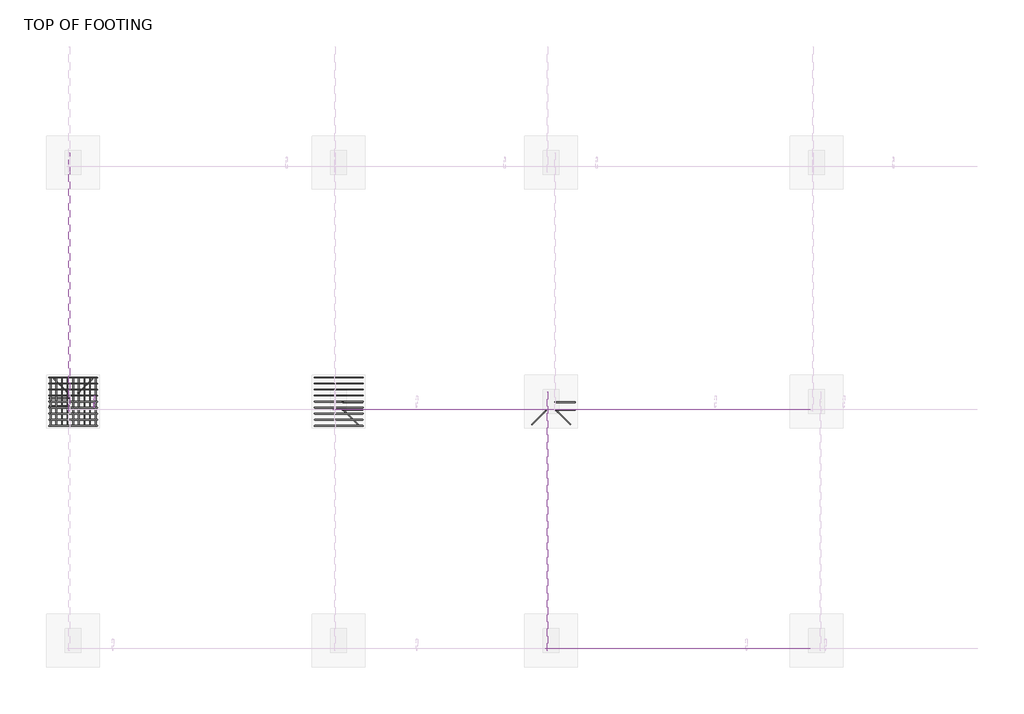
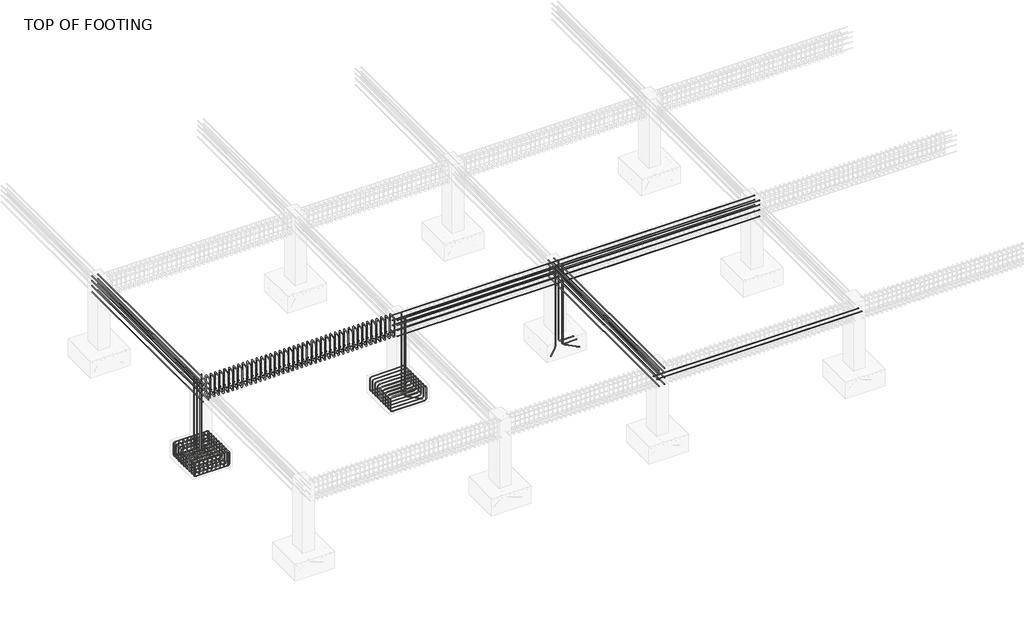
# One storey, part 4 of 13: 32 reinforcing bars.
"""IFC4 building model written with IfcOpenShell, lengths in millimetres."""

from ifc_helpers import new_model, si_unit, point, frame, origin, place, context, project, spatial, polyline, circle_curve, trimmed, segment, composite_curve, source, transform, mapped, element, save
from ifc_brep_helpers import swept_disk

model = new_model("IFC4")

# Units and contexts
model_context = context("Model", 3, world=origin())
ifc_project = project(units=[si_unit("LENGTHUNIT", "METRE", prefix="MILLI")], contexts=[model_context])

# Site, building, storey
site = spatial("IfcSite", under=ifc_project)
building = spatial("IfcBuilding", under=site)
storey = spatial("IfcBuildingStorey", under=building, Name="TOP OF FOOTING", Elevation=-1828.8)

# Reinforcing bars
placement = place(None, origin())
reinforcing_bar_shape = source(origin(), model_context, "Body", "SolidModel", [
    swept_disk(composite_curve([segment(polyline([(-12666.6498378, 8486.1851908, -2049.322685), (-12666.6498378, 8486.1851908, -2196.622685)]), True, "CONTINUOUS"), segment(trimmed(circle_curve(frame((-12712.9998378, 8486.1851908, -2196.622685), z_axis=(0.0, 1.0, 0.0), x_axis=(46.350000000000364, 0.0, 0.0)), 46.35), [point((-12666.6498378, 8486.1851908, -2196.622685))], [point((-12712.9998378, 8486.1851908, -2242.972685))], True, "CARTESIAN"), True, "CONTINUOUS"), segment(polyline([(-12712.9998378, 8486.1851908, -2242.972685), (-13527.5998378, 8486.1851908, -2242.972685)]), True, "CONTINUOUS"), segment(trimmed(circle_curve(frame((-13527.5998378, 8486.1851908, -2196.622685), z_axis=(0.0, 1.0, 0.0), x_axis=(0.0, 0.0, -46.350000000000364)), 46.35), [point((-13527.5998378, 8486.1851908, -2242.972685))], [point((-13573.9498378, 8486.1851908, -2196.622685))], True, "CARTESIAN"), True, "CONTINUOUS"), segment(polyline([(-13573.9498378, 8486.1851908, -2196.622685), (-13573.9498378, 8486.1851908, -2049.322685)]), True, "CONTINUOUS")], self_intersect=False), 6.35),
])
element("IfcReinforcingBar", 1, at=placement, inside=storey, context=model_context, shape_type="MappedRepresentation", body=[
    mapped(reinforcing_bar_shape, transform((0.0, 0.0, 0.0), x_axis=(1.0, 0.0, 0.0), y_axis=(0.0, 1.0, 0.0), z_axis=(0.0, 0.0, 1.0))),
    mapped(reinforcing_bar_shape, transform((0.0, -113.4125, 0.0), x_axis=(1.0, 0.0, 0.0), y_axis=(0.0, 1.0, 0.0), z_axis=(0.0, 0.0, 1.0))),
    mapped(reinforcing_bar_shape, transform((0.0, -226.825, 0.0), x_axis=(1.0, 0.0, 0.0), y_axis=(0.0, 1.0, 0.0), z_axis=(0.0, 0.0, 1.0))),
    mapped(reinforcing_bar_shape, transform((0.0, -340.2375, 0.0), x_axis=(1.0, 0.0, 0.0), y_axis=(0.0, 1.0, 0.0), z_axis=(0.0, 0.0, 1.0))),
    mapped(reinforcing_bar_shape, transform((0.0, -453.65, 0.0), x_axis=(1.0, 0.0, 0.0), y_axis=(0.0, 1.0, 0.0), z_axis=(0.0, 0.0, 1.0))),
    mapped(reinforcing_bar_shape, transform((0.0, -567.0625, 0.0), x_axis=(1.0, 0.0, 0.0), y_axis=(0.0, 1.0, 0.0), z_axis=(0.0, 0.0, 1.0))),
    mapped(reinforcing_bar_shape, transform((0.0, -680.475, 0.0), x_axis=(1.0, 0.0, 0.0), y_axis=(0.0, 1.0, 0.0), z_axis=(0.0, 0.0, 1.0))),
    mapped(reinforcing_bar_shape, transform((0.0, -793.8875, 0.0), x_axis=(1.0, 0.0, 0.0), y_axis=(0.0, 1.0, 0.0), z_axis=(0.0, 0.0, 1.0))),
    mapped(reinforcing_bar_shape, transform((0.0, -907.3, 0.0), x_axis=(1.0, 0.0, 0.0), y_axis=(0.0, 1.0, 0.0), z_axis=(0.0, 0.0, 1.0))),
])
reinforcing_bar_2_shape = source(origin(), model_context, "Body", "SolidModel", [
    swept_disk(composite_curve([segment(polyline([(-13573.9498378, 8486.1851908, -2051.3998363), (-13573.9498378, 8486.1851908, -1904.0998363)]), True, "CONTINUOUS"), segment(trimmed(circle_curve(frame((-13527.5998378, 8486.1851908, -1904.0998363), z_axis=(0.0, 1.0, 0.0), x_axis=(-46.350000000000364, 0.0, 0.0)), 46.35), [point((-13573.9498378, 8486.1851908, -1904.0998363))], [point((-13527.5998378, 8486.1851908, -1857.7498363))], True, "CARTESIAN"), True, "CONTINUOUS"), segment(polyline([(-13527.5998378, 8486.1851908, -1857.7498363), (-12712.9998378, 8486.1851908, -1857.7498363)]), True, "CONTINUOUS"), segment(trimmed(circle_curve(frame((-12712.9998378, 8486.1851908, -1904.0998363), z_axis=(0.0, 1.0, 0.0), x_axis=(0.0, 0.0, 46.350000000000136)), 46.35), [point((-12712.9998378, 8486.1851908, -1857.7498363))], [point((-12666.6498378, 8486.1851908, -1904.0998363))], True, "CARTESIAN"), True, "CONTINUOUS"), segment(polyline([(-12666.6498378, 8486.1851908, -1904.0998363), (-12666.6498378, 8486.1851908, -2051.3998363)]), True, "CONTINUOUS")], self_intersect=False), 6.35),
])
element("IfcReinforcingBar", 2, at=placement, inside=storey, context=model_context, shape_type="MappedRepresentation", body=[
    mapped(reinforcing_bar_2_shape, transform((0.0, 0.0, 0.0), x_axis=(1.0, 0.0, 0.0), y_axis=(0.0, 1.0, 0.0), z_axis=(0.0, 0.0, 1.0))),
    mapped(reinforcing_bar_2_shape, transform((0.0, -113.4125, 0.0), x_axis=(1.0, 0.0, 0.0), y_axis=(0.0, 1.0, 0.0), z_axis=(0.0, 0.0, 1.0))),
    mapped(reinforcing_bar_2_shape, transform((0.0, -226.825, 0.0), x_axis=(1.0, 0.0, 0.0), y_axis=(0.0, 1.0, 0.0), z_axis=(0.0, 0.0, 1.0))),
    mapped(reinforcing_bar_2_shape, transform((0.0, -340.2375, 0.0), x_axis=(1.0, 0.0, 0.0), y_axis=(0.0, 1.0, 0.0), z_axis=(0.0, 0.0, 1.0))),
    mapped(reinforcing_bar_2_shape, transform((0.0, -453.65, 0.0), x_axis=(1.0, 0.0, 0.0), y_axis=(0.0, 1.0, 0.0), z_axis=(0.0, 0.0, 1.0))),
    mapped(reinforcing_bar_2_shape, transform((0.0, -567.0625, 0.0), x_axis=(1.0, 0.0, 0.0), y_axis=(0.0, 1.0, 0.0), z_axis=(0.0, 0.0, 1.0))),
    mapped(reinforcing_bar_2_shape, transform((0.0, -680.475, 0.0), x_axis=(1.0, 0.0, 0.0), y_axis=(0.0, 1.0, 0.0), z_axis=(0.0, 0.0, 1.0))),
    mapped(reinforcing_bar_2_shape, transform((0.0, -793.8875, 0.0), x_axis=(1.0, 0.0, 0.0), y_axis=(0.0, 1.0, 0.0), z_axis=(0.0, 0.0, 1.0))),
    mapped(reinforcing_bar_2_shape, transform((0.0, -907.3, 0.0), x_axis=(1.0, 0.0, 0.0), y_axis=(0.0, 1.0, 0.0), z_axis=(0.0, 0.0, 1.0))),
])
reinforcing_bar_3_shape = source(origin(), model_context, "Body", "SolidModel", [
    swept_disk(composite_curve([segment(polyline([(-13542.4641345, 8486.1851908, -2025.081839), (-13542.4641345, 8486.1851908, -2172.381839)]), True, "CONTINUOUS"), segment(trimmed(circle_curve(frame((-13542.4641345, 8439.8351908, -2172.381839), z_axis=(-1.0, 0.0, 0.0), x_axis=(0.0, 46.350000000000364, 0.0)), 46.35), [point((-13542.4641345, 8486.1851908, -2172.381839))], [point((-13542.4641345, 8439.8351908, -2218.731839))], True, "CARTESIAN"), True, "CONTINUOUS"), segment(polyline([(-13542.4641345, 8439.8351908, -2218.731839), (-13542.4641345, 7625.2351908, -2218.731839)]), True, "CONTINUOUS"), segment(trimmed(circle_curve(frame((-13542.4641345, 7625.2351908, -2172.381839), z_axis=(-1.0, 0.0, 0.0), x_axis=(0.0, 0.0, -46.34999999999991)), 46.35), [point((-13542.4641345, 7625.2351908, -2218.731839))], [point((-13542.4641345, 7578.8851908, -2172.381839))], True, "CARTESIAN"), True, "CONTINUOUS"), segment(polyline([(-13542.4641345, 7578.8851908, -2172.381839), (-13542.4641345, 7578.8851908, -2025.081839)]), True, "CONTINUOUS")], self_intersect=False), 6.35),
])
element("IfcReinforcingBar", 3, at=placement, inside=storey, context=model_context, shape_type="MappedRepresentation", body=[
    mapped(reinforcing_bar_3_shape, transform((0.0, 0.0, 0.0), x_axis=(1.0, 0.0, 0.0), y_axis=(0.0, 1.0, 0.0), z_axis=(0.0, 0.0, 1.0))),
    mapped(reinforcing_bar_3_shape, transform((105.924033, 0.0, 0.0), x_axis=(1.0, 0.0, 0.0), y_axis=(0.0, 1.0, 0.0), z_axis=(0.0, 0.0, 1.0))),
    mapped(reinforcing_bar_3_shape, transform((211.8480661, 0.0, 0.0), x_axis=(1.0, 0.0, 0.0), y_axis=(0.0, 1.0, 0.0), z_axis=(0.0, 0.0, 1.0))),
    mapped(reinforcing_bar_3_shape, transform((317.7720991, 0.0, 0.0), x_axis=(1.0, 0.0, 0.0), y_axis=(0.0, 1.0, 0.0), z_axis=(0.0, 0.0, 1.0))),
    mapped(reinforcing_bar_3_shape, transform((423.6961321, 0.0, 0.0), x_axis=(1.0, 0.0, 0.0), y_axis=(0.0, 1.0, 0.0), z_axis=(0.0, 0.0, 1.0))),
    mapped(reinforcing_bar_3_shape, transform((529.6201652, 0.0, 0.0), x_axis=(1.0, 0.0, 0.0), y_axis=(0.0, 1.0, 0.0), z_axis=(0.0, 0.0, 1.0))),
    mapped(reinforcing_bar_3_shape, transform((635.5441982, 0.0, 0.0), x_axis=(1.0, 0.0, 0.0), y_axis=(0.0, 1.0, 0.0), z_axis=(0.0, 0.0, 1.0))),
    mapped(reinforcing_bar_3_shape, transform((741.4682312, 0.0, 0.0), x_axis=(1.0, 0.0, 0.0), y_axis=(0.0, 1.0, 0.0), z_axis=(0.0, 0.0, 1.0))),
    mapped(reinforcing_bar_3_shape, transform((847.3922643, 0.0, 0.0), x_axis=(1.0, 0.0, 0.0), y_axis=(0.0, 1.0, 0.0), z_axis=(0.0, 0.0, 1.0))),
])
reinforcing_bar_4_shape = source(origin(), model_context, "Body", "SolidModel", [
    swept_disk(composite_curve([segment(polyline([(-12695.0718702, 8486.1851908, -2069.0990329), (-12695.0718702, 8486.1851908, -1921.7990329)]), True, "CONTINUOUS"), segment(trimmed(circle_curve(frame((-12695.0718702, 8439.8351908, -1921.7990329), z_axis=(1.0, 0.0, 0.0), x_axis=(0.0, 46.350000000000364, 0.0)), 46.35), [point((-12695.0718702, 8486.1851908, -1921.7990329))], [point((-12695.0718702, 8439.8351908, -1875.4490329))], True, "CARTESIAN"), True, "CONTINUOUS"), segment(polyline([(-12695.0718702, 8439.8351908, -1875.4490329), (-12695.0718702, 7625.2351908, -1875.4490329)]), True, "CONTINUOUS"), segment(trimmed(circle_curve(frame((-12695.0718702, 7625.2351908, -1921.7990329), z_axis=(1.0, 0.0, 0.0), x_axis=(0.0, 0.0, 46.34999999999991)), 46.35), [point((-12695.0718702, 7625.2351908, -1875.4490329))], [point((-12695.0718702, 7578.8851908, -1921.7990329))], True, "CARTESIAN"), True, "CONTINUOUS"), segment(polyline([(-12695.0718702, 7578.8851908, -1921.7990329), (-12695.0718702, 7578.8851908, -2069.0990329)]), True, "CONTINUOUS")], self_intersect=False), 6.35),
])
element("IfcReinforcingBar", 4, at=placement, inside=storey, context=model_context, shape_type="MappedRepresentation", body=[
    mapped(reinforcing_bar_4_shape, transform((0.0, 0.0, 0.0), x_axis=(1.0, 0.0, 0.0), y_axis=(0.0, 1.0, 0.0), z_axis=(0.0, 0.0, 1.0))),
    mapped(reinforcing_bar_4_shape, transform((-105.924033, 0.0, 0.0), x_axis=(1.0, 0.0, 0.0), y_axis=(0.0, 1.0, 0.0), z_axis=(0.0, 0.0, 1.0))),
    mapped(reinforcing_bar_4_shape, transform((-211.8480661, 0.0, 0.0), x_axis=(1.0, 0.0, 0.0), y_axis=(0.0, 1.0, 0.0), z_axis=(0.0, 0.0, 1.0))),
    mapped(reinforcing_bar_4_shape, transform((-317.7720991, 0.0, 0.0), x_axis=(1.0, 0.0, 0.0), y_axis=(0.0, 1.0, 0.0), z_axis=(0.0, 0.0, 1.0))),
    mapped(reinforcing_bar_4_shape, transform((-423.6961321, 0.0, 0.0), x_axis=(1.0, 0.0, 0.0), y_axis=(0.0, 1.0, 0.0), z_axis=(0.0, 0.0, 1.0))),
    mapped(reinforcing_bar_4_shape, transform((-529.6201652, 0.0, 0.0), x_axis=(1.0, 0.0, 0.0), y_axis=(0.0, 1.0, 0.0), z_axis=(0.0, 0.0, 1.0))),
    mapped(reinforcing_bar_4_shape, transform((-635.5441982, 0.0, 0.0), x_axis=(1.0, 0.0, 0.0), y_axis=(0.0, 1.0, 0.0), z_axis=(0.0, 0.0, 1.0))),
    mapped(reinforcing_bar_4_shape, transform((-741.4682312, 0.0, 0.0), x_axis=(1.0, 0.0, 0.0), y_axis=(0.0, 1.0, 0.0), z_axis=(0.0, 0.0, 1.0))),
    mapped(reinforcing_bar_4_shape, transform((-847.3922643, 0.0, 0.0), x_axis=(1.0, 0.0, 0.0), y_axis=(0.0, 1.0, 0.0), z_axis=(0.0, 0.0, 1.0))),
])
reinforcing_bar_5_shape = source(origin(), model_context, "Body", "SolidModel", [
    swept_disk(composite_curve([segment(polyline([(-7666.6498378, 8486.1851908, -2049.322685), (-7666.6498378, 8486.1851908, -2196.622685)]), True, "CONTINUOUS"), segment(trimmed(circle_curve(frame((-7712.9998378, 8486.1851908, -2196.622685), z_axis=(0.0, 1.0, 0.0), x_axis=(46.350000000000364, 0.0, 0.0)), 46.35), [point((-7666.6498378, 8486.1851908, -2196.622685))], [point((-7712.9998378, 8486.1851908, -2242.972685))], True, "CARTESIAN"), True, "CONTINUOUS"), segment(polyline([(-7712.9998378, 8486.1851908, -2242.972685), (-8527.5998378, 8486.1851908, -2242.972685)]), True, "CONTINUOUS"), segment(trimmed(circle_curve(frame((-8527.5998378, 8486.1851908, -2196.622685), z_axis=(0.0, 1.0, 0.0), x_axis=(0.0, 0.0, -46.350000000000364)), 46.35), [point((-8527.5998378, 8486.1851908, -2242.972685))], [point((-8573.9498378, 8486.1851908, -2196.622685))], True, "CARTESIAN"), True, "CONTINUOUS"), segment(polyline([(-8573.9498378, 8486.1851908, -2196.622685), (-8573.9498378, 8486.1851908, -2049.322685)]), True, "CONTINUOUS")], self_intersect=False), 6.35),
])
element("IfcReinforcingBar", 5, at=placement, inside=storey, context=model_context, shape_type="MappedRepresentation", body=[
    mapped(reinforcing_bar_5_shape, transform((0.0, 0.0, 0.0), x_axis=(1.0, 0.0, 0.0), y_axis=(0.0, 1.0, 0.0), z_axis=(0.0, 0.0, 1.0))),
    mapped(reinforcing_bar_5_shape, transform((0.0, -113.4125, 0.0), x_axis=(1.0, 0.0, 0.0), y_axis=(0.0, 1.0, 0.0), z_axis=(0.0, 0.0, 1.0))),
    mapped(reinforcing_bar_5_shape, transform((0.0, -226.825, 0.0), x_axis=(1.0, 0.0, 0.0), y_axis=(0.0, 1.0, 0.0), z_axis=(0.0, 0.0, 1.0))),
    mapped(reinforcing_bar_5_shape, transform((0.0, -340.2375, 0.0), x_axis=(1.0, 0.0, 0.0), y_axis=(0.0, 1.0, 0.0), z_axis=(0.0, 0.0, 1.0))),
    mapped(reinforcing_bar_5_shape, transform((0.0, -453.65, 0.0), x_axis=(1.0, 0.0, 0.0), y_axis=(0.0, 1.0, 0.0), z_axis=(0.0, 0.0, 1.0))),
    mapped(reinforcing_bar_5_shape, transform((0.0, -567.0625, 0.0), x_axis=(1.0, 0.0, 0.0), y_axis=(0.0, 1.0, 0.0), z_axis=(0.0, 0.0, 1.0))),
    mapped(reinforcing_bar_5_shape, transform((0.0, -680.475, 0.0), x_axis=(1.0, 0.0, 0.0), y_axis=(0.0, 1.0, 0.0), z_axis=(0.0, 0.0, 1.0))),
    mapped(reinforcing_bar_5_shape, transform((0.0, -793.8875, 0.0), x_axis=(1.0, 0.0, 0.0), y_axis=(0.0, 1.0, 0.0), z_axis=(0.0, 0.0, 1.0))),
    mapped(reinforcing_bar_5_shape, transform((0.0, -907.3, 0.0), x_axis=(1.0, 0.0, 0.0), y_axis=(0.0, 1.0, 0.0), z_axis=(0.0, 0.0, 1.0))),
])
reinforcing_bar_6_shape = source(origin(), model_context, "Body", "SolidModel", [
    swept_disk(composite_curve([segment(polyline([(-8573.9498378, 8486.1851908, -2051.3998363), (-8573.9498378, 8486.1851908, -1904.0998363)]), True, "CONTINUOUS"), segment(trimmed(circle_curve(frame((-8527.5998378, 8486.1851908, -1904.0998363), z_axis=(0.0, 1.0, 0.0), x_axis=(-46.350000000000364, 0.0, 0.0)), 46.35), [point((-8573.9498378, 8486.1851908, -1904.0998363))], [point((-8527.5998378, 8486.1851908, -1857.7498363))], True, "CARTESIAN"), True, "CONTINUOUS"), segment(polyline([(-8527.5998378, 8486.1851908, -1857.7498363), (-7712.9998378, 8486.1851908, -1857.7498363)]), True, "CONTINUOUS"), segment(trimmed(circle_curve(frame((-7712.9998378, 8486.1851908, -1904.0998363), z_axis=(0.0, 1.0, 0.0), x_axis=(0.0, 0.0, 46.350000000000136)), 46.35), [point((-7712.9998378, 8486.1851908, -1857.7498363))], [point((-7666.6498378, 8486.1851908, -1904.0998363))], True, "CARTESIAN"), True, "CONTINUOUS"), segment(polyline([(-7666.6498378, 8486.1851908, -1904.0998363), (-7666.6498378, 8486.1851908, -2051.3998363)]), True, "CONTINUOUS")], self_intersect=False), 6.35),
])
element("IfcReinforcingBar", 6, at=placement, inside=storey, context=model_context, shape_type="MappedRepresentation", body=[
    mapped(reinforcing_bar_6_shape, transform((0.0, 0.0, 0.0), x_axis=(1.0, 0.0, 0.0), y_axis=(0.0, 1.0, 0.0), z_axis=(0.0, 0.0, 1.0))),
    mapped(reinforcing_bar_6_shape, transform((0.0, -113.4125, 0.0), x_axis=(1.0, 0.0, 0.0), y_axis=(0.0, 1.0, 0.0), z_axis=(0.0, 0.0, 1.0))),
    mapped(reinforcing_bar_6_shape, transform((0.0, -226.825, 0.0), x_axis=(1.0, 0.0, 0.0), y_axis=(0.0, 1.0, 0.0), z_axis=(0.0, 0.0, 1.0))),
    mapped(reinforcing_bar_6_shape, transform((0.0, -340.2375, 0.0), x_axis=(1.0, 0.0, 0.0), y_axis=(0.0, 1.0, 0.0), z_axis=(0.0, 0.0, 1.0))),
    mapped(reinforcing_bar_6_shape, transform((0.0, -453.65, 0.0), x_axis=(1.0, 0.0, 0.0), y_axis=(0.0, 1.0, 0.0), z_axis=(0.0, 0.0, 1.0))),
    mapped(reinforcing_bar_6_shape, transform((0.0, -567.0625, 0.0), x_axis=(1.0, 0.0, 0.0), y_axis=(0.0, 1.0, 0.0), z_axis=(0.0, 0.0, 1.0))),
    mapped(reinforcing_bar_6_shape, transform((0.0, -680.475, 0.0), x_axis=(1.0, 0.0, 0.0), y_axis=(0.0, 1.0, 0.0), z_axis=(0.0, 0.0, 1.0))),
    mapped(reinforcing_bar_6_shape, transform((0.0, -793.8875, 0.0), x_axis=(1.0, 0.0, 0.0), y_axis=(0.0, 1.0, 0.0), z_axis=(0.0, 0.0, 1.0))),
    mapped(reinforcing_bar_6_shape, transform((0.0, -907.3, 0.0), x_axis=(1.0, 0.0, 0.0), y_axis=(0.0, 1.0, 0.0), z_axis=(0.0, 0.0, 1.0))),
])
reinforcing_bar_7_shape = source(origin(), model_context, "Body", "SolidModel", [
    swept_disk(composite_curve([segment(polyline([(-4044.6810723, 8023.2621018, -40.0), (-4044.6810723, 8023.2621018, -2147.4714407)]), True, "CONTINUOUS"), segment(trimmed(circle_curve(frame((-3998.3310723, 8023.2621018, -2147.4714407), z_axis=(0.0, -1.0, 0.0), x_axis=(-46.34999999999991, 0.0, 0.0)), 46.35), [point((-4044.6810723, 8023.2621018, -2147.4714407))], [point((-3998.3310723, 8023.2621018, -2193.8214407))], True, "CARTESIAN"), True, "CONTINUOUS"), segment(polyline([(-3998.3310723, 8023.2621018, -2193.8214407), (-3667.4997506, 8023.2621018, -2193.8214407)]), True, "CONTINUOUS")], self_intersect=False), 6.35),
])
element("IfcReinforcingBar", 7, at=placement, inside=storey, context=model_context, shape_type="MappedRepresentation", body=[
    mapped(reinforcing_bar_7_shape, transform((0.0, 0.0, 0.0), x_axis=(1.0, 0.0, 0.0), y_axis=(0.0, 1.0, 0.0), z_axis=(0.0, 0.0, 1.0))),
    mapped(reinforcing_bar_7_shape, transform((0.0, -144.620853, 0.0), x_axis=(1.0, 0.0, 0.0), y_axis=(0.0, 1.0, 0.0), z_axis=(0.0, 0.0, 1.0))),
])
element("IfcReinforcingBar", 8, at=placement, inside=storey, context=model_context, shape_type="SolidModel", body=[
    swept_disk(composite_curve([segment(polyline([(-4024.6810723, 7868.8851908, -40.0), (-4024.6810723, 7868.8851908, -2147.4714407)]), True, "CONTINUOUS"), segment(trimmed(circle_curve(frame((-3991.906673, 7836.1107915, -2147.4714407), z_axis=(-0.7071067811865542, -0.7071067811865408, 0.0), x_axis=(-32.774399299999914, 32.77439929999946, 0.0)), 46.35), [point((-4024.6810723, 7868.8851908, -2147.4714407))], [point((-3991.906673, 7836.1107915, -2193.8214407))], True, "CARTESIAN"), True, "CONTINUOUS"), segment(polyline([(-3991.906673, 7836.1107915, -2193.8214407), (-3757.973602, 7602.1777205, -2193.8214407)]), True, "CONTINUOUS")], self_intersect=False), 6.35),
])
element("IfcReinforcingBar", 9, at=placement, inside=storey, context=model_context, shape_type="SolidModel", body=[
    swept_disk(composite_curve([segment(polyline([(-4215.9186034, 7868.8851908, -40.0), (-4215.9186034, 7868.8851908, -2147.4714407)]), True, "CONTINUOUS"), segment(trimmed(circle_curve(frame((-4248.6930027, 7836.1107915, -2147.4714407), z_axis=(-0.7071067811865339, 0.7071067811865611, 0.0), x_axis=(32.77439929999946, 32.77439929999946, 0.0)), 46.35), [point((-4215.9186034, 7868.8851908, -2147.4714407))], [point((-4248.6930027, 7836.1107915, -2193.8214407))], True, "CARTESIAN"), True, "CONTINUOUS"), segment(polyline([(-4248.6930027, 7836.1107915, -2193.8214407), (-4482.6260737, 7602.1777205, -2193.8214407)]), True, "CONTINUOUS")], self_intersect=False), 6.35),
])
reinforcing_bar_8_shape = source(origin(), model_context, "Body", "SolidModel", [
    swept_disk(composite_curve([segment(polyline([(-8044.6810723, 8023.2621018, -40.0), (-8044.6810723, 8023.2621018, -2147.4714407)]), True, "CONTINUOUS"), segment(trimmed(circle_curve(frame((-7998.3310723, 8023.2621018, -2147.4714407), z_axis=(0.0, -1.0, 0.0), x_axis=(-46.349999999999454, 0.0, 0.0)), 46.35), [point((-8044.6810723, 8023.2621018, -2147.4714407))], [point((-7998.3310723, 8023.2621018, -2193.8214407))], True, "CARTESIAN"), True, "CONTINUOUS"), segment(polyline([(-7998.3310723, 8023.2621018, -2193.8214407), (-7667.4997506, 8023.2621018, -2193.8214407)]), True, "CONTINUOUS")], self_intersect=False), 6.35),
])
element("IfcReinforcingBar", 10, at=placement, inside=storey, context=model_context, shape_type="MappedRepresentation", body=[
    mapped(reinforcing_bar_8_shape, transform((0.0, 0.0, 0.0), x_axis=(1.0, 0.0, 0.0), y_axis=(0.0, 1.0, 0.0), z_axis=(0.0, 0.0, 1.0))),
    mapped(reinforcing_bar_8_shape, transform((0.0, -144.620853, 0.0), x_axis=(1.0, 0.0, 0.0), y_axis=(0.0, 1.0, 0.0), z_axis=(0.0, 0.0, 1.0))),
])
element("IfcReinforcingBar", 11, at=placement, inside=storey, context=model_context, shape_type="SolidModel", body=[
    swept_disk(composite_curve([segment(polyline([(-8024.6810723, 7868.8851908, -40.0), (-8024.6810723, 7868.8851908, -2147.4714407)]), True, "CONTINUOUS"), segment(trimmed(circle_curve(frame((-7991.906673, 7836.1107915, -2147.4714407), z_axis=(-0.7071067811865542, -0.7071067811865408, 0.0), x_axis=(-32.77439929999946, 32.77439929999946, 0.0)), 46.35), [point((-8024.6810723, 7868.8851908, -2147.4714407))], [point((-7991.906673, 7836.1107915, -2193.8214407))], True, "CARTESIAN"), True, "CONTINUOUS"), segment(polyline([(-7991.906673, 7836.1107915, -2193.8214407), (-7757.973602, 7602.1777205, -2193.8214407)]), True, "CONTINUOUS")], self_intersect=False), 6.35),
])
element("IfcReinforcingBar", 12, at=placement, inside=storey, context=model_context, shape_type="SolidModel", body=[
    swept_disk(composite_curve([segment(polyline([(-13024.6810723, 8196.1851908, -40.0), (-13024.6810723, 8196.1851908, -2147.4714407)]), True, "CONTINUOUS"), segment(trimmed(circle_curve(frame((-12991.906673, 8228.9595901, -2147.4714407), z_axis=(0.7071067811865476, -0.7071067811865475, 0.0), x_axis=(-32.77439930000037, -32.77439929999855, 0.0)), 46.35), [point((-13024.6810723, 8196.1851908, -2147.4714407))], [point((-12991.906673, 8228.9595901, -2193.8214407))], True, "CARTESIAN"), True, "CONTINUOUS"), segment(polyline([(-12991.906673, 8228.9595901, -2193.8214407), (-12757.973602, 8462.8926611, -2193.8214407)]), True, "CONTINUOUS")], self_intersect=False), 6.35),
])
element("IfcReinforcingBar", 13, at=placement, inside=storey, context=model_context, shape_type="SolidModel", body=[
    swept_disk(composite_curve([segment(polyline([(-13215.9186034, 8196.1851908, -40.0), (-13215.9186034, 8196.1851908, -2147.4714407)]), True, "CONTINUOUS"), segment(trimmed(circle_curve(frame((-13248.6930027, 8228.9595901, -2147.4714407), z_axis=(0.7071067811865679, 0.7071067811865271, 0.0), x_axis=(32.77439930000037, -32.77439929999855, 0.0)), 46.35), [point((-13215.9186034, 8196.1851908, -2147.4714407))], [point((-13248.6930027, 8228.9595901, -2193.8214407))], True, "CARTESIAN"), True, "CONTINUOUS"), segment(polyline([(-13248.6930027, 8228.9595901, -2193.8214407), (-13482.6260737, 8462.8926611, -2193.8214407)]), True, "CONTINUOUS")], self_intersect=False), 6.35),
])
reinforcing_bar_9_shape = source(origin(), model_context, "Body", "SolidModel", [
    swept_disk(composite_curve([segment(polyline([(-13195.9186034, 8098.2621018, -40.0), (-13195.9186034, 8098.2621018, -2147.4714407)]), True, "CONTINUOUS"), segment(trimmed(circle_curve(frame((-13242.2686034, 8098.2621018, -2147.4714407), z_axis=(0.0, 1.0, 0.0), x_axis=(46.350000000000364, 0.0, 0.0)), 46.35), [point((-13195.9186034, 8098.2621018, -2147.4714407))], [point((-13242.2686034, 8098.2621018, -2193.8214407))], True, "CARTESIAN"), True, "CONTINUOUS"), segment(polyline([(-13242.2686034, 8098.2621018, -2193.8214407), (-13573.0999251, 8098.2621018, -2193.8214407)]), True, "CONTINUOUS")], self_intersect=False), 6.35),
])
element("IfcReinforcingBar", 14, at=placement, inside=storey, context=model_context, shape_type="MappedRepresentation", body=[
    mapped(reinforcing_bar_9_shape, transform((0.0, 0.0, 0.0), x_axis=(1.0, 0.0, 0.0), y_axis=(0.0, 1.0, 0.0), z_axis=(0.0, 0.0, 1.0))),
    mapped(reinforcing_bar_9_shape, transform((0.0, -144.620853, 0.0), x_axis=(1.0, 0.0, 0.0), y_axis=(0.0, 1.0, 0.0), z_axis=(0.0, 0.0, 1.0))),
])
reinforcing_bar_10_shape = source(origin(), model_context, "Body", "SolidModel", [
    swept_disk(composite_curve([segment(polyline([(-4192.6754021, 3347.5351908, -87.6047527), (-4192.6754021, 8217.5351908, -87.6047527)]), True, "CONTINUOUS")], self_intersect=False), 6.35),
])
element("IfcReinforcingBar", 15, at=placement, inside=storey, context=model_context, shape_type="MappedRepresentation", body=[
    mapped(reinforcing_bar_10_shape, transform((0.0, 0.0, 0.0), x_axis=(1.0, 0.0, 0.0), y_axis=(0.0, 1.0, 0.0), z_axis=(0.0, 0.0, 1.0))),
    mapped(reinforcing_bar_10_shape, transform((144.710816, 0.0, 0.0), x_axis=(1.0, 0.0, 0.0), y_axis=(0.0, 1.0, 0.0), z_axis=(0.0, 0.0, 1.0))),
])
reinforcing_bar_11_shape = source(origin(), model_context, "Body", "SolidModel", [
    swept_disk(composite_curve([segment(polyline([(-4192.6754021, 3347.5351908, -212.6047527), (-4192.6754021, 8217.5351908, -212.6047527)]), True, "CONTINUOUS")], self_intersect=False), 6.35),
])
element("IfcReinforcingBar", 16, at=placement, inside=storey, context=model_context, shape_type="MappedRepresentation", body=[
    mapped(reinforcing_bar_11_shape, transform((0.0, 0.0, 0.0), x_axis=(1.0, 0.0, 0.0), y_axis=(0.0, 1.0, 0.0), z_axis=(0.0, 0.0, 1.0))),
    mapped(reinforcing_bar_11_shape, transform((144.710816, 0.0, 0.0), x_axis=(1.0, 0.0, 0.0), y_axis=(0.0, 1.0, 0.0), z_axis=(0.0, 0.0, 1.0))),
])
reinforcing_bar_12_shape = source(origin(), model_context, "Body", "SolidModel", [
    swept_disk(composite_curve([segment(polyline([(-4192.6754021, 3347.5351908, -517.6047527), (-4192.6754021, 8217.5351908, -517.6047527)]), True, "CONTINUOUS")], self_intersect=False), 6.35),
])
element("IfcReinforcingBar", 17, at=placement, inside=storey, context=model_context, shape_type="MappedRepresentation", body=[
    mapped(reinforcing_bar_12_shape, transform((0.0, 0.0, 0.0), x_axis=(1.0, 0.0, 0.0), y_axis=(0.0, 1.0, 0.0), z_axis=(0.0, 0.0, 1.0))),
    mapped(reinforcing_bar_12_shape, transform((144.710816, 0.0, 0.0), x_axis=(1.0, 0.0, 0.0), y_axis=(0.0, 1.0, 0.0), z_axis=(0.0, 0.0, 1.0))),
])
reinforcing_bar_13_shape = source(origin(), model_context, "Body", "SolidModel", [
    swept_disk(composite_curve([segment(polyline([(-4192.6754021, 3347.5351908, -347.6047527), (-4192.6754021, 8217.5351908, -347.6047527)]), True, "CONTINUOUS")], self_intersect=False), 6.35),
])
element("IfcReinforcingBar", 18, at=placement, inside=storey, context=model_context, shape_type="MappedRepresentation", body=[
    mapped(reinforcing_bar_13_shape, transform((0.0, 0.0, 0.0), x_axis=(1.0, 0.0, 0.0), y_axis=(0.0, 1.0, 0.0), z_axis=(0.0, 0.0, 1.0))),
    mapped(reinforcing_bar_13_shape, transform((144.710816, 0.0, 0.0), x_axis=(1.0, 0.0, 0.0), y_axis=(0.0, 1.0, 0.0), z_axis=(0.0, 0.0, 1.0))),
])
reinforcing_bar_14_shape = source(origin(), model_context, "Body", "SolidModel", [
    swept_disk(composite_curve([segment(polyline([(-13192.6754021, 7847.5351908, -87.6047527), (-13192.6754021, 12717.5351908, -87.6047527)]), True, "CONTINUOUS")], self_intersect=False), 6.35),
])
element("IfcReinforcingBar", 19, at=placement, inside=storey, context=model_context, shape_type="MappedRepresentation", body=[
    mapped(reinforcing_bar_14_shape, transform((0.0, 0.0, 0.0), x_axis=(1.0, 0.0, 0.0), y_axis=(0.0, 1.0, 0.0), z_axis=(0.0, 0.0, 1.0))),
    mapped(reinforcing_bar_14_shape, transform((144.710816, 0.0, 0.0), x_axis=(1.0, 0.0, 0.0), y_axis=(0.0, 1.0, 0.0), z_axis=(0.0, 0.0, 1.0))),
])
reinforcing_bar_15_shape = source(origin(), model_context, "Body", "SolidModel", [
    swept_disk(composite_curve([segment(polyline([(-13192.6754021, 7847.5351908, -212.6047527), (-13192.6754021, 12717.5351908, -212.6047527)]), True, "CONTINUOUS")], self_intersect=False), 6.35),
])
element("IfcReinforcingBar", 20, at=placement, inside=storey, context=model_context, shape_type="MappedRepresentation", body=[
    mapped(reinforcing_bar_15_shape, transform((0.0, 0.0, 0.0), x_axis=(1.0, 0.0, 0.0), y_axis=(0.0, 1.0, 0.0), z_axis=(0.0, 0.0, 1.0))),
    mapped(reinforcing_bar_15_shape, transform((144.710816, 0.0, 0.0), x_axis=(1.0, 0.0, 0.0), y_axis=(0.0, 1.0, 0.0), z_axis=(0.0, 0.0, 1.0))),
])
reinforcing_bar_16_shape = source(origin(), model_context, "Body", "SolidModel", [
    swept_disk(composite_curve([segment(polyline([(-13192.6754021, 7847.5351908, -517.6047527), (-13192.6754021, 12717.5351908, -517.6047527)]), True, "CONTINUOUS")], self_intersect=False), 6.35),
])
element("IfcReinforcingBar", 21, at=placement, inside=storey, context=model_context, shape_type="MappedRepresentation", body=[
    mapped(reinforcing_bar_16_shape, transform((0.0, 0.0, 0.0), x_axis=(1.0, 0.0, 0.0), y_axis=(0.0, 1.0, 0.0), z_axis=(0.0, 0.0, 1.0))),
    mapped(reinforcing_bar_16_shape, transform((144.710816, 0.0, 0.0), x_axis=(1.0, 0.0, 0.0), y_axis=(0.0, 1.0, 0.0), z_axis=(0.0, 0.0, 1.0))),
])
reinforcing_bar_17_shape = source(origin(), model_context, "Body", "SolidModel", [
    swept_disk(composite_curve([segment(polyline([(-13192.6754021, 7847.5351908, -347.6047527), (-13192.6754021, 12717.5351908, -347.6047527)]), True, "CONTINUOUS")], self_intersect=False), 6.35),
])
element("IfcReinforcingBar", 22, at=placement, inside=storey, context=model_context, shape_type="MappedRepresentation", body=[
    mapped(reinforcing_bar_17_shape, transform((0.0, 0.0, 0.0), x_axis=(1.0, 0.0, 0.0), y_axis=(0.0, 1.0, 0.0), z_axis=(0.0, 0.0, 1.0))),
    mapped(reinforcing_bar_17_shape, transform((144.710816, 0.0, 0.0), x_axis=(1.0, 0.0, 0.0), y_axis=(0.0, 1.0, 0.0), z_axis=(0.0, 0.0, 1.0))),
])
reinforcing_bar_18_shape = source(origin(), model_context, "Body", "SolidModel", [
    swept_disk(composite_curve([segment(polyline([(-8276.6498378, 8071.2594254, -444.3886395), (-8276.6498378, 8127.0029884, -500.1322024)]), True, "CONTINUOUS"), segment(trimmed(circle_curve(frame((-8276.6498378, 8104.8351908, -522.3), z_axis=(-1.0, 0.0, 0.0), x_axis=(0.0, 22.167797599999176, 22.16779759999997)), 31.35), [point((-8276.6498378, 8127.0029884, -500.1322024))], [point((-8276.6498378, 8104.8351908, -553.65))], True, "CARTESIAN"), True, "CONTINUOUS"), segment(polyline([(-8276.6498378, 8104.8351908, -553.65), (-8276.6498378, 7960.2351908, -553.65)]), True, "CONTINUOUS"), segment(trimmed(circle_curve(frame((-8276.6498378, 7960.2351908, -522.3), z_axis=(-1.0, 0.0, 0.0), x_axis=(0.0, 0.0, -31.350000000000023)), 31.35), [point((-8276.6498378, 7960.2351908, -553.65))], [point((-8276.6498378, 7928.8851908, -522.3))], True, "CARTESIAN"), True, "CONTINUOUS"), segment(polyline([(-8276.6498378, 7928.8851908, -522.3), (-8276.6498378, 7928.8851908, -77.7)]), True, "CONTINUOUS"), segment(trimmed(circle_curve(frame((-8274.7328097, 7960.1765235, -77.7), z_axis=(-0.9981286353368323, 0.061149221750018364, 0.0), x_axis=(-1.917028099998788, -31.291332700000567, 0.0)), 31.35), [point((-8276.6498378, 7928.8851908, -77.7))], [point((-8274.7328097, 7960.1765235, -46.35))], True, "CARTESIAN"), True, "CONTINUOUS"), segment(polyline([(-8274.7328097, 7960.1765235, -46.35), (-8265.8668659, 8104.8938581, -46.35)]), True, "CONTINUOUS"), segment(trimmed(circle_curve(frame((-8265.8668659, 8104.8938581, -77.7), z_axis=(-0.9981286353368323, 0.061149221750018364, 0.0), x_axis=(0.0, 0.0, 31.35)), 31.35), [point((-8265.8668659, 8104.8938581, -46.35))], [point((-8263.9498378, 8136.1851908, -77.7))], True, "CARTESIAN"), True, "CONTINUOUS"), segment(polyline([(-8263.9498378, 8136.1851908, -77.7), (-8263.9498378, 8136.1851908, -522.3)]), True, "CONTINUOUS"), segment(trimmed(circle_curve(frame((-8263.9498378, 8104.8351908, -522.3), z_axis=(-1.0, 0.0, 0.0), x_axis=(0.0, 31.349999999999454, 0.0)), 31.35), [point((-8263.9498378, 8136.1851908, -522.3))], [point((-8263.9498378, 8082.6673932, -544.4677976))], True, "CARTESIAN"), True, "CONTINUOUS"), segment(polyline([(-8263.9498378, 8082.6673932, -544.4677976), (-8263.9498378, 8026.9238303, -488.7242346)]), True, "CONTINUOUS")], self_intersect=False), 6.35),
])
element("IfcReinforcingBar", 23, at=placement, inside=storey, context=model_context, shape_type="MappedRepresentation", body=[
    mapped(reinforcing_bar_18_shape, transform((0.0, 0.0, 0.0), x_axis=(1.0, 0.0, 0.0), y_axis=(0.0, 1.0, 0.0), z_axis=(0.0, 0.0, 1.0))),
    mapped(reinforcing_bar_18_shape, transform((-117.1825, 0.0, 0.0), x_axis=(1.0, 0.0, 0.0), y_axis=(0.0, 1.0, 0.0), z_axis=(0.0, 0.0, 1.0))),
    mapped(reinforcing_bar_18_shape, transform((-234.365, 0.0, 0.0), x_axis=(1.0, 0.0, 0.0), y_axis=(0.0, 1.0, 0.0), z_axis=(0.0, 0.0, 1.0))),
    mapped(reinforcing_bar_18_shape, transform((-351.5475, 0.0, 0.0), x_axis=(1.0, 0.0, 0.0), y_axis=(0.0, 1.0, 0.0), z_axis=(0.0, 0.0, 1.0))),
    mapped(reinforcing_bar_18_shape, transform((-468.73, 0.0, 0.0), x_axis=(1.0, 0.0, 0.0), y_axis=(0.0, 1.0, 0.0), z_axis=(0.0, 0.0, 1.0))),
    mapped(reinforcing_bar_18_shape, transform((-585.9125, 0.0, 0.0), x_axis=(1.0, 0.0, 0.0), y_axis=(0.0, 1.0, 0.0), z_axis=(0.0, 0.0, 1.0))),
    mapped(reinforcing_bar_18_shape, transform((-703.095, 0.0, 0.0), x_axis=(1.0, 0.0, 0.0), y_axis=(0.0, 1.0, 0.0), z_axis=(0.0, 0.0, 1.0))),
    mapped(reinforcing_bar_18_shape, transform((-820.2775, 0.0, 0.0), x_axis=(1.0, 0.0, 0.0), y_axis=(0.0, 1.0, 0.0), z_axis=(0.0, 0.0, 1.0))),
    mapped(reinforcing_bar_18_shape, transform((-937.46, 0.0, 0.0), x_axis=(1.0, 0.0, 0.0), y_axis=(0.0, 1.0, 0.0), z_axis=(0.0, 0.0, 1.0))),
    mapped(reinforcing_bar_18_shape, transform((-1054.6425, 0.0, 0.0), x_axis=(1.0, 0.0, 0.0), y_axis=(0.0, 1.0, 0.0), z_axis=(0.0, 0.0, 1.0))),
    mapped(reinforcing_bar_18_shape, transform((-1171.825, 0.0, 0.0), x_axis=(1.0, 0.0, 0.0), y_axis=(0.0, 1.0, 0.0), z_axis=(0.0, 0.0, 1.0))),
    mapped(reinforcing_bar_18_shape, transform((-1289.0075, 0.0, 0.0), x_axis=(1.0, 0.0, 0.0), y_axis=(0.0, 1.0, 0.0), z_axis=(0.0, 0.0, 1.0))),
    mapped(reinforcing_bar_18_shape, transform((-1406.19, 0.0, 0.0), x_axis=(1.0, 0.0, 0.0), y_axis=(0.0, 1.0, 0.0), z_axis=(0.0, 0.0, 1.0))),
    mapped(reinforcing_bar_18_shape, transform((-1523.3725, 0.0, 0.0), x_axis=(1.0, 0.0, 0.0), y_axis=(0.0, 1.0, 0.0), z_axis=(0.0, 0.0, 1.0))),
    mapped(reinforcing_bar_18_shape, transform((-1640.555, 0.0, 0.0), x_axis=(1.0, 0.0, 0.0), y_axis=(0.0, 1.0, 0.0), z_axis=(0.0, 0.0, 1.0))),
    mapped(reinforcing_bar_18_shape, transform((-1757.7375, 0.0, 0.0), x_axis=(1.0, 0.0, 0.0), y_axis=(0.0, 1.0, 0.0), z_axis=(0.0, 0.0, 1.0))),
    mapped(reinforcing_bar_18_shape, transform((-1874.92, 0.0, 0.0), x_axis=(1.0, 0.0, 0.0), y_axis=(0.0, 1.0, 0.0), z_axis=(0.0, 0.0, 1.0))),
    mapped(reinforcing_bar_18_shape, transform((-1992.1025, 0.0, 0.0), x_axis=(1.0, 0.0, 0.0), y_axis=(0.0, 1.0, 0.0), z_axis=(0.0, 0.0, 1.0))),
    mapped(reinforcing_bar_18_shape, transform((-2109.285, 0.0, 0.0), x_axis=(1.0, 0.0, 0.0), y_axis=(0.0, 1.0, 0.0), z_axis=(0.0, 0.0, 1.0))),
    mapped(reinforcing_bar_18_shape, transform((-2226.4675, 0.0, 0.0), x_axis=(1.0, 0.0, 0.0), y_axis=(0.0, 1.0, 0.0), z_axis=(0.0, 0.0, 1.0))),
    mapped(reinforcing_bar_18_shape, transform((-2343.65, 0.0, 0.0), x_axis=(1.0, 0.0, 0.0), y_axis=(0.0, 1.0, 0.0), z_axis=(0.0, 0.0, 1.0))),
    mapped(reinforcing_bar_18_shape, transform((-2460.8325, 0.0, 0.0), x_axis=(1.0, 0.0, 0.0), y_axis=(0.0, 1.0, 0.0), z_axis=(0.0, 0.0, 1.0))),
    mapped(reinforcing_bar_18_shape, transform((-2578.015, 0.0, 0.0), x_axis=(1.0, 0.0, 0.0), y_axis=(0.0, 1.0, 0.0), z_axis=(0.0, 0.0, 1.0))),
    mapped(reinforcing_bar_18_shape, transform((-2695.1975, 0.0, 0.0), x_axis=(1.0, 0.0, 0.0), y_axis=(0.0, 1.0, 0.0), z_axis=(0.0, 0.0, 1.0))),
    mapped(reinforcing_bar_18_shape, transform((-2812.38, 0.0, 0.0), x_axis=(1.0, 0.0, 0.0), y_axis=(0.0, 1.0, 0.0), z_axis=(0.0, 0.0, 1.0))),
    mapped(reinforcing_bar_18_shape, transform((-2929.5625, 0.0, 0.0), x_axis=(1.0, 0.0, 0.0), y_axis=(0.0, 1.0, 0.0), z_axis=(0.0, 0.0, 1.0))),
    mapped(reinforcing_bar_18_shape, transform((-3046.745, 0.0, 0.0), x_axis=(1.0, 0.0, 0.0), y_axis=(0.0, 1.0, 0.0), z_axis=(0.0, 0.0, 1.0))),
    mapped(reinforcing_bar_18_shape, transform((-3163.9275, 0.0, 0.0), x_axis=(1.0, 0.0, 0.0), y_axis=(0.0, 1.0, 0.0), z_axis=(0.0, 0.0, 1.0))),
    mapped(reinforcing_bar_18_shape, transform((-3281.11, 0.0, 0.0), x_axis=(1.0, 0.0, 0.0), y_axis=(0.0, 1.0, 0.0), z_axis=(0.0, 0.0, 1.0))),
    mapped(reinforcing_bar_18_shape, transform((-3398.2925, 0.0, 0.0), x_axis=(1.0, 0.0, 0.0), y_axis=(0.0, 1.0, 0.0), z_axis=(0.0, 0.0, 1.0))),
    mapped(reinforcing_bar_18_shape, transform((-3515.475, 0.0, 0.0), x_axis=(1.0, 0.0, 0.0), y_axis=(0.0, 1.0, 0.0), z_axis=(0.0, 0.0, 1.0))),
    mapped(reinforcing_bar_18_shape, transform((-3632.6575, 0.0, 0.0), x_axis=(1.0, 0.0, 0.0), y_axis=(0.0, 1.0, 0.0), z_axis=(0.0, 0.0, 1.0))),
    mapped(reinforcing_bar_18_shape, transform((-3749.84, 0.0, 0.0), x_axis=(1.0, 0.0, 0.0), y_axis=(0.0, 1.0, 0.0), z_axis=(0.0, 0.0, 1.0))),
    mapped(reinforcing_bar_18_shape, transform((-3867.0225, 0.0, 0.0), x_axis=(1.0, 0.0, 0.0), y_axis=(0.0, 1.0, 0.0), z_axis=(0.0, 0.0, 1.0))),
    mapped(reinforcing_bar_18_shape, transform((-3984.205, 0.0, 0.0), x_axis=(1.0, 0.0, 0.0), y_axis=(0.0, 1.0, 0.0), z_axis=(0.0, 0.0, 1.0))),
    mapped(reinforcing_bar_18_shape, transform((-4101.3875, 0.0, 0.0), x_axis=(1.0, 0.0, 0.0), y_axis=(0.0, 1.0, 0.0), z_axis=(0.0, 0.0, 1.0))),
    mapped(reinforcing_bar_18_shape, transform((-4218.57, 0.0, 0.0), x_axis=(1.0, 0.0, 0.0), y_axis=(0.0, 1.0, 0.0), z_axis=(0.0, 0.0, 1.0))),
    mapped(reinforcing_bar_18_shape, transform((-4335.7525, 0.0, 0.0), x_axis=(1.0, 0.0, 0.0), y_axis=(0.0, 1.0, 0.0), z_axis=(0.0, 0.0, 1.0))),
    mapped(reinforcing_bar_18_shape, transform((-4452.935, 0.0, 0.0), x_axis=(1.0, 0.0, 0.0), y_axis=(0.0, 1.0, 0.0), z_axis=(0.0, 0.0, 1.0))),
    mapped(reinforcing_bar_18_shape, transform((-4570.1175, 0.0, 0.0), x_axis=(1.0, 0.0, 0.0), y_axis=(0.0, 1.0, 0.0), z_axis=(0.0, 0.0, 1.0))),
    mapped(reinforcing_bar_18_shape, transform((-4687.3, 0.0, 0.0), x_axis=(1.0, 0.0, 0.0), y_axis=(0.0, 1.0, 0.0), z_axis=(0.0, 0.0, 1.0))),
])
reinforcing_bar_19_shape = source(origin(), model_context, "Body", "SolidModel", [
    swept_disk(composite_curve([segment(polyline([(-4010.2998378, 7885.1596265, -87.6047527), (-8230.2998378, 7885.1596265, -87.6047527)]), True, "CONTINUOUS")], self_intersect=False), 6.35),
])
element("IfcReinforcingBar", 24, at=placement, inside=storey, context=model_context, shape_type="MappedRepresentation", body=[
    mapped(reinforcing_bar_19_shape, transform((0.0, 0.0, 0.0), x_axis=(1.0, 0.0, 0.0), y_axis=(0.0, 1.0, 0.0), z_axis=(0.0, 0.0, 1.0))),
    mapped(reinforcing_bar_19_shape, transform((0.0, 219.710816, 0.0), x_axis=(1.0, 0.0, 0.0), y_axis=(0.0, 1.0, 0.0), z_axis=(0.0, 0.0, 1.0))),
])
reinforcing_bar_20_shape = source(origin(), model_context, "Body", "SolidModel", [
    swept_disk(composite_curve([segment(polyline([(-4010.2998378, 7885.1596265, -212.6047527), (-8230.2998378, 7885.1596265, -212.6047527)]), True, "CONTINUOUS")], self_intersect=False), 6.35),
])
element("IfcReinforcingBar", 25, at=placement, inside=storey, context=model_context, shape_type="MappedRepresentation", body=[
    mapped(reinforcing_bar_20_shape, transform((0.0, 0.0, 0.0), x_axis=(1.0, 0.0, 0.0), y_axis=(0.0, 1.0, 0.0), z_axis=(0.0, 0.0, 1.0))),
    mapped(reinforcing_bar_20_shape, transform((0.0, 219.710816, 0.0), x_axis=(1.0, 0.0, 0.0), y_axis=(0.0, 1.0, 0.0), z_axis=(0.0, 0.0, 1.0))),
])
reinforcing_bar_21_shape = source(origin(), model_context, "Body", "SolidModel", [
    swept_disk(composite_curve([segment(polyline([(-4010.2998378, 7885.1596265, -517.6047527), (-8230.2998378, 7885.1596265, -517.6047527)]), True, "CONTINUOUS")], self_intersect=False), 6.35),
])
element("IfcReinforcingBar", 26, at=placement, inside=storey, context=model_context, shape_type="MappedRepresentation", body=[
    mapped(reinforcing_bar_21_shape, transform((0.0, 0.0, 0.0), x_axis=(1.0, 0.0, 0.0), y_axis=(0.0, 1.0, 0.0), z_axis=(0.0, 0.0, 1.0))),
    mapped(reinforcing_bar_21_shape, transform((0.0, 219.710816, 0.0), x_axis=(1.0, 0.0, 0.0), y_axis=(0.0, 1.0, 0.0), z_axis=(0.0, 0.0, 1.0))),
])
reinforcing_bar_22_shape = source(origin(), model_context, "Body", "SolidModel", [
    swept_disk(composite_curve([segment(polyline([(-4010.2998378, 7885.1596265, -347.6047527), (-8230.2998378, 7885.1596265, -347.6047527)]), True, "CONTINUOUS")], self_intersect=False), 6.35),
])
element("IfcReinforcingBar", 27, at=placement, inside=storey, context=model_context, shape_type="MappedRepresentation", body=[
    mapped(reinforcing_bar_22_shape, transform((0.0, 0.0, 0.0), x_axis=(1.0, 0.0, 0.0), y_axis=(0.0, 1.0, 0.0), z_axis=(0.0, 0.0, 1.0))),
    mapped(reinforcing_bar_22_shape, transform((0.0, 219.710816, 0.0), x_axis=(1.0, 0.0, 0.0), y_axis=(0.0, 1.0, 0.0), z_axis=(0.0, 0.0, 1.0))),
])
reinforcing_bar_23_shape = source(origin(), model_context, "Body", "SolidModel", [
    swept_disk(composite_curve([segment(polyline([(989.7001622, 7885.1596265, -87.6047527), (-4230.2998378, 7885.1596265, -87.6047527)]), True, "CONTINUOUS")], self_intersect=False), 6.35),
])
element("IfcReinforcingBar", 28, at=placement, inside=storey, context=model_context, shape_type="MappedRepresentation", body=[
    mapped(reinforcing_bar_23_shape, transform((0.0, 0.0, 0.0), x_axis=(1.0, 0.0, 0.0), y_axis=(0.0, 1.0, 0.0), z_axis=(0.0, 0.0, 1.0))),
    mapped(reinforcing_bar_23_shape, transform((0.0, 219.710816, 0.0), x_axis=(1.0, 0.0, 0.0), y_axis=(0.0, 1.0, 0.0), z_axis=(0.0, 0.0, 1.0))),
])
reinforcing_bar_24_shape = source(origin(), model_context, "Body", "SolidModel", [
    swept_disk(composite_curve([segment(polyline([(989.7001622, 7885.1596265, -212.6047527), (-4230.2998378, 7885.1596265, -212.6047527)]), True, "CONTINUOUS")], self_intersect=False), 6.35),
])
element("IfcReinforcingBar", 29, at=placement, inside=storey, context=model_context, shape_type="MappedRepresentation", body=[
    mapped(reinforcing_bar_24_shape, transform((0.0, 0.0, 0.0), x_axis=(1.0, 0.0, 0.0), y_axis=(0.0, 1.0, 0.0), z_axis=(0.0, 0.0, 1.0))),
    mapped(reinforcing_bar_24_shape, transform((0.0, 219.710816, 0.0), x_axis=(1.0, 0.0, 0.0), y_axis=(0.0, 1.0, 0.0), z_axis=(0.0, 0.0, 1.0))),
])
reinforcing_bar_25_shape = source(origin(), model_context, "Body", "SolidModel", [
    swept_disk(composite_curve([segment(polyline([(989.7001622, 7885.1596265, -517.6047527), (-4230.2998378, 7885.1596265, -517.6047527)]), True, "CONTINUOUS")], self_intersect=False), 6.35),
])
element("IfcReinforcingBar", 30, at=placement, inside=storey, context=model_context, shape_type="MappedRepresentation", body=[
    mapped(reinforcing_bar_25_shape, transform((0.0, 0.0, 0.0), x_axis=(1.0, 0.0, 0.0), y_axis=(0.0, 1.0, 0.0), z_axis=(0.0, 0.0, 1.0))),
    mapped(reinforcing_bar_25_shape, transform((0.0, 219.710816, 0.0), x_axis=(1.0, 0.0, 0.0), y_axis=(0.0, 1.0, 0.0), z_axis=(0.0, 0.0, 1.0))),
])
reinforcing_bar_26_shape = source(origin(), model_context, "Body", "SolidModel", [
    swept_disk(composite_curve([segment(polyline([(989.7001622, 7885.1596265, -347.6047527), (-4230.2998378, 7885.1596265, -347.6047527)]), True, "CONTINUOUS")], self_intersect=False), 6.35),
])
element("IfcReinforcingBar", 31, at=placement, inside=storey, context=model_context, shape_type="MappedRepresentation", body=[
    mapped(reinforcing_bar_26_shape, transform((0.0, 0.0, 0.0), x_axis=(1.0, 0.0, 0.0), y_axis=(0.0, 1.0, 0.0), z_axis=(0.0, 0.0, 1.0))),
    mapped(reinforcing_bar_26_shape, transform((0.0, 219.710816, 0.0), x_axis=(1.0, 0.0, 0.0), y_axis=(0.0, 1.0, 0.0), z_axis=(0.0, 0.0, 1.0))),
])
reinforcing_bar_27_shape = source(origin(), model_context, "Body", "SolidModel", [
    swept_disk(composite_curve([segment(polyline([(989.7001622, 3385.1596265, -347.6047527), (-4230.2998378, 3385.1596265, -347.6047527)]), True, "CONTINUOUS")], self_intersect=False), 6.35),
])
element("IfcReinforcingBar", 32, at=placement, inside=storey, context=model_context, shape_type="MappedRepresentation", body=[
    mapped(reinforcing_bar_27_shape, transform((0.0, 0.0, 0.0), x_axis=(1.0, 0.0, 0.0), y_axis=(0.0, 1.0, 0.0), z_axis=(0.0, 0.0, 1.0))),
    mapped(reinforcing_bar_27_shape, transform((0.0, 144.710816, 0.0), x_axis=(1.0, 0.0, 0.0), y_axis=(0.0, 1.0, 0.0), z_axis=(0.0, 0.0, 1.0))),
])

save(model, "model.ifc")

# Revit data of these elements
# Elements 1, 2, 3, 4, 5, 6, 7, 8, 9, 10, 11, 12, 13, 14, 15, 16, 17, 18, 19, 20, 21, 22, 23, 24, 25, 26, 27, 28, 29, 30, 31, 32 (IfcReinforcingBar)
#   Phase Created = New Construction
